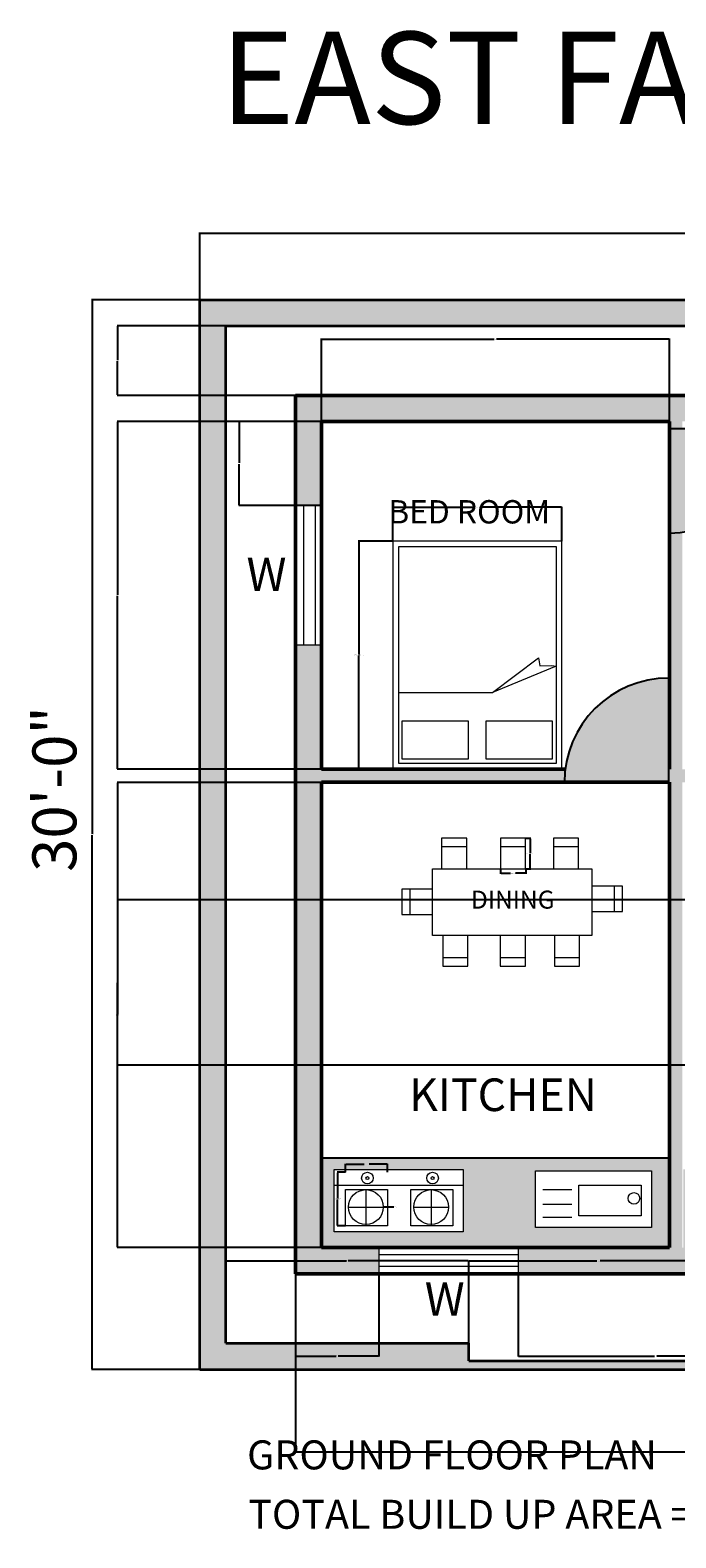
# Model space of a CAD drawing. Units: inches. Extents: x -48 to 546, y -53 to 467.
# Tile 1 of 3: x -48 to 174, y -53 to 467. Entities that reach past the tile are written whole.
import ezdxf

# ---------------------------------------------------------------- set-up
doc = ezdxf.new("R2010")
doc.units = ezdxf.units.IN
doc.header["$MEASUREMENT"] = 0
for name, color, linetype, lineweight in [('A-ANNO-DIMS', 2, 'Continuous', 18), ('A-ANNO-TEXT', 7, 'Continuous', 18), ('A-AREA-IDEN', 7, 'Continuous', 25), ('A-DOOR', 4, 'Continuous', 25), ('A-EQPM', 8, 'Continuous', 18), ('A-FLOR-CASE', 8, 'Continuous', 25), ('A-FLOR-FIXT', 9, 'Continuous', 18), ('A-FURN', 8, 'Continuous', 18), ('A-GLAZ', 4, 'Continuous', 18), ('A-WALL', 7, 'Continuous', 50), ('C-PROP', 7, 'Continuous', 35)]:
    doc.layers.add(name, color=color, linetype=linetype, lineweight=lineweight)
for name, color, linetype, lineweight, true_color in [('A-FLOR-PATT', 253, 'Continuous', 13, 0x9898cc), ('A-WALL-PATT', 251, 'Continuous', 13, 0x636466), ('C-PROP-PATT', 251, 'Continuous', 13, 0x636466)]:
    doc.layers.add(name, color=color, linetype=linetype, lineweight=lineweight, true_color=true_color)
doc.styles.get("Standard").update_dxf_attribs({"font": 'arial.ttf'})
doc.dimstyles.get("Standard").update_dxf_attribs({"dimtxt": 0.18, "dimasz": 0.18, "dimexe": 0.18, "dimexo": 0.0625, "dimgap": 0.09, "dimtad": 0, "dimtih": 1, "dimtoh": 1, "dimdec": 4, "dimzin": 0, "dimdsep": 46, "dimtxsty": 'Standard', "dimcen": 0.09, "dimadec": 0, "dimazin": 0, "dimtfac": 1, "dimtdec": 4, "dimtofl": 0, "dimtmove": 0, "dimatfit": 3, "dimfxl": 1, "dimtolj": 1, "dimtzin": 0, "dimarcsym": 0})

# ---------------------------------------------------------------- blocks, each defined once
blk = doc.blocks.new('*D3')
at = {"layer": 'A-ANNO-DIMS', "color": 0, "lineweight": -2, "transparency": 16777216}
for p, q in [((10.2, 374.58), (10.2, 397.68)), ((10.38, 397.5), (254.09, 397.5)), ((499.02, 397.5), (255.31, 397.5)), ((499.2, 374.58), (499.2, 397.68))]:
    blk.add_line(p, q, dxfattribs=at)
at = {"layer": 'A-ANNO-DIMS', "color": 0, "transparency": 16777216}
for points in [[(10.38, 397.53), (10.38, 397.47), (10.2, 397.5)], [(499.02, 397.53), (499.02, 397.47), (499.2, 397.5)]]:
    blk.add_solid(points, dxfattribs=at)
at = {"layer": 'Defpoints', "color": 0, "transparency": 16777216}
for p in [(499.2, 397.5), (10.2, 374.51), (499.2, 374.51)]:
    blk.add_point(p, dxfattribs=at)
at = {"layer": 'A-ANNO-DIMS', "color": 0, "transparency": 16777216, "insert": (254.7, 397.5), "char_height": 0.18, "width": 0.9058, "attachment_point": 5}
blk.add_mtext('\\A1;489.0000', dxfattribs=at)
blk = doc.blocks.new('*D4')
at = {"layer": 'A-ANNO-DIMS', "color": 0, "lineweight": -2, "transparency": 16777216}
for p, q in [((10.14, 374.51), (-27.18, 374.51)), ((-27, 374.33), (-27, 190.2)), ((-27, 5.69), (-27, 189.83)), ((10.14, 5.51), (-27.18, 5.51))]:
    blk.add_line(p, q, dxfattribs=at)
at = {"layer": 'A-ANNO-DIMS', "color": 0, "transparency": 16777216}
for points in [[(-27.03, 374.33), (-26.97, 374.33), (-27, 374.51)], [(-27.03, 5.69), (-26.97, 5.69), (-27, 5.51)]]:
    blk.add_solid(points, dxfattribs=at)
at = {"layer": 'Defpoints', "color": 0, "transparency": 16777216}
for p in [(10.2, 374.51), (-27, 5.51), (10.2, 5.51)]:
    blk.add_point(p, dxfattribs=at)
at = {"layer": 'A-ANNO-DIMS', "color": 0, "transparency": 16777216, "insert": (-27, 190.01), "char_height": 0.18, "attachment_point": 5}
blk.add_mtext('\\A1;369.0000', dxfattribs=at)
blk = doc.blocks.new('DOOR-SWING-36IN')
for p, q in [((0, 36), (0, 0)), ((0, 0), (36, 0))]:
    blk.add_line(p, q)
blk.add_arc((0, 0), 36, 0, 90)
blk = doc.blocks.new('CHAIR-DINING')
blk.add_line((0.01, 7.68), (8.69, 7.68))
blk.add_lwpolyline([(0, 0), (8.68, 0), (8.68, 10.53), (0, 10.53)], close=True)
blk = doc.blocks.new('BED-DOUBLE')
for p, q in [((34.35, 26.2), (50.2, 38.16)), ((50.2, 38.16), (50.65, 35.43)), ((56.35, 35.37), (34.37, 26.2)), ((50.65, 35.43), (54.7, 35.6)), ((1.91, 26.2), (34.35, 26.2))]:
    blk.add_line(p, q)
for points in [[(0, 0), (58.3, 0), (58.3, 78.39), (0, 78.39)], [(1.9, 1.9), (56.4, 1.9), (56.4, 76.49), (1.9, 76.49)], [(3.12, 3.4), (26.1, 3.4), (26.1, 16.4), (3.12, 16.4)], [(32.03, 3.4), (55.02, 3.4), (55.02, 16.4), (32.03, 16.4)]]:
    blk.add_lwpolyline(points, close=True)
blk = doc.blocks.new('WIN-48IN-FRONT')
for p, q in [((0, 9), (0, 0)), ((48, 6.49), (0, 6.49)), ((48, 9), (48, 0)), ((48, 2.49), (0, 2.49)), ((48, 2.49), (0, 2.49)), ((48, 2.49), (0, 2.49))]:
    blk.add_line(p, q)
blk = doc.blocks.new('WIN-48IN-BEDROOM')
for p, q in [((0, 48), (9, 48)), ((2.8, 48), (2.8, 0)), ((6.8, 48), (6.8, 0)), ((6.8, 48), (6.8, 0)), ((6.8, 48), (6.8, 0)), ((0, 0), (9, 0))]:
    blk.add_line(p, q)
blk = doc.blocks.new('COOKTOP-BURNER')
for p, q in [((7, 12.5), (7, 0)), ((1, 6.5), (13, 6.5))]:
    blk.add_line(p, q)
blk.add_lwpolyline([(0, 12.5), (14.5, 12.5), (14.5, 0), (0, 0)], close=True)
for centre, radius in [((7.5, 16.5), 2), ((7.5, 16.5), 0.5), ((7, 6.5), 6)]:
    blk.add_circle(centre, radius)
blk = doc.blocks.new('*D12')
at = {"layer": 'A-ANNO-DIMS', "color": 0, "lineweight": -2, "transparency": 16777216}
for p, q in [((76.76, 291.15), (64.88, 291.15)), ((65.06, 290.97), (65.06, 252.14)), ((65.06, 212.94), (65.06, 251.77)), ((76.76, 212.76), (64.88, 212.76))]:
    blk.add_line(p, q, dxfattribs=at)
at = {"layer": 'A-ANNO-DIMS', "color": 0, "transparency": 16777216}
for points in [[(65.03, 290.97), (65.09, 290.97), (65.06, 291.15)], [(65.03, 212.94), (65.09, 212.94), (65.06, 212.76)]]:
    blk.add_solid(points, dxfattribs=at)
at = {"layer": 'Defpoints', "color": 0, "transparency": 16777216}
for p in [(65.06, 291.15), (76.82, 291.15), (76.82, 212.76)]:
    blk.add_point(p, dxfattribs=at)
at = {"layer": 'A-ANNO-DIMS', "color": 0, "transparency": 16777216, "insert": (65.06, 251.95), "char_height": 0.18, "attachment_point": 5}
blk.add_mtext('\\A1;DOUBLE BED 6\'-6 1/2" TYP.', dxfattribs=at)
blk = doc.blocks.new('*D13')
at = {"layer": 'A-ANNO-DIMS', "color": 0, "lineweight": -2, "transparency": 16777216}
for p, q in [((76.82, 291.21), (76.82, 303.09)), ((77, 302.91), (105.05, 302.91)), ((134.94, 302.91), (106.89, 302.91)), ((135.12, 291.21), (135.12, 303.09))]:
    blk.add_line(p, q, dxfattribs=at)
at = {"layer": 'A-ANNO-DIMS', "color": 0, "transparency": 16777216}
for points in [[(77, 302.94), (77, 302.88), (76.82, 302.91)], [(134.94, 302.94), (134.94, 302.88), (135.12, 302.91)]]:
    blk.add_solid(points, dxfattribs=at)
at = {"layer": 'Defpoints', "color": 0, "transparency": 16777216}
for p in [(135.12, 302.91), (76.82, 291.15), (135.12, 291.15)]:
    blk.add_point(p, dxfattribs=at)
at = {"layer": 'A-ANNO-DIMS', "color": 0, "transparency": 16777216, "insert": (105.97, 302.91), "char_height": 0.18, "attachment_point": 5}
blk.add_mtext('\\A1;4\'-10 1/2" TYP.', dxfattribs=at)
blk = doc.blocks.new('*D22')
at = {"layer": 'A-ANNO-DIMS', "color": 0, "lineweight": -2, "transparency": 16777216}
for p, q in [((122.69, 188.75), (124.38, 188.75)), ((124.2, 188.57), (124.2, 183.67)), ((124.2, 178.4), (124.2, 183.3)), ((122.69, 178.22), (124.38, 178.22))]:
    blk.add_line(p, q, dxfattribs=at)
at = {"layer": 'A-ANNO-DIMS', "color": 0, "transparency": 16777216}
for points in [[(124.17, 188.57), (124.23, 188.57), (124.2, 188.75)], [(124.17, 178.4), (124.23, 178.4), (124.2, 178.22)]]:
    blk.add_solid(points, dxfattribs=at)
at = {"layer": 'Defpoints', "color": 0, "transparency": 16777216}
for p in [(122.63, 188.75), (124.2, 188.75), (122.63, 178.22)]:
    blk.add_point(p, dxfattribs=at)
at = {"layer": 'A-ANNO-DIMS', "color": 0, "transparency": 16777216, "insert": (124.2, 183.48), "char_height": 0.18, "attachment_point": 5}
blk.add_mtext('\\A1;CHAIR 0\'-10 1/2" TYP.', dxfattribs=at)
blk = doc.blocks.new('*D23')
at = {"layer": 'A-ANNO-DIMS', "color": 0, "lineweight": -2, "transparency": 16777216}
for p, q in [((113.94, 178.16), (113.94, 176.46)), ((122.63, 178.16), (122.63, 176.46)), ((114.12, 176.64), (117.43, 176.64)), ((122.45, 176.64), (119.13, 176.64))]:
    blk.add_line(p, q, dxfattribs=at)
at = {"layer": 'A-ANNO-DIMS', "color": 0, "transparency": 16777216}
for points in [[(114.12, 176.67), (114.12, 176.61), (113.94, 176.64)], [(122.45, 176.67), (122.45, 176.61), (122.63, 176.64)]]:
    blk.add_solid(points, dxfattribs=at)
at = {"layer": 'Defpoints', "color": 0, "transparency": 16777216}
for p in [(113.94, 178.22), (122.63, 178.22), (122.63, 176.64)]:
    blk.add_point(p, dxfattribs=at)
at = {"layer": 'A-ANNO-DIMS', "color": 0, "transparency": 16777216, "insert": (118.28, 176.64), "char_height": 0.18, "attachment_point": 5}
blk.add_mtext('\\A1;0\'-8 1/2" TYP.', dxfattribs=at)
blk = doc.blocks.new('*D24')
at = {"layer": 'A-ANNO-DIMS', "color": 0, "lineweight": -2, "transparency": 16777216}
for p, q in [((60.44, 73.5), (57.55, 73.5)), ((57.73, 73.32), (57.73, 64.43)), ((57.73, 55.18), (57.73, 64.07)), ((60.44, 55), (57.55, 55))]:
    blk.add_line(p, q, dxfattribs=at)
at = {"layer": 'A-ANNO-DIMS', "color": 0, "transparency": 16777216}
for points in [[(57.7, 73.32), (57.76, 73.32), (57.73, 73.5)], [(57.7, 55.18), (57.76, 55.18), (57.73, 55)]]:
    blk.add_solid(points, dxfattribs=at)
at = {"layer": 'Defpoints', "color": 0, "transparency": 16777216}
for p in [(57.73, 73.5), (60.5, 73.5), (60.5, 55)]:
    blk.add_point(p, dxfattribs=at)
at = {"layer": 'A-ANNO-DIMS', "color": 0, "transparency": 16777216, "insert": (57.73, 64.25), "char_height": 0.18, "attachment_point": 5}
blk.add_mtext('\\A1;BURNER 1\'-6 1/2" TYP.', dxfattribs=at)
blk = doc.blocks.new('*D25')
at = {"layer": 'A-ANNO-DIMS', "color": 0, "lineweight": -2, "transparency": 16777216}
for p, q in [((60.5, 73.56), (60.5, 76.46)), ((60.68, 76.28), (66.91, 76.28)), ((74.82, 76.28), (68.59, 76.28)), ((75, 73.56), (75, 76.46))]:
    blk.add_line(p, q, dxfattribs=at)
at = {"layer": 'A-ANNO-DIMS', "color": 0, "transparency": 16777216}
for points in [[(60.68, 76.31), (60.68, 76.25), (60.5, 76.28)], [(74.82, 76.31), (74.82, 76.25), (75, 76.28)]]:
    blk.add_solid(points, dxfattribs=at)
at = {"layer": 'Defpoints', "color": 0, "transparency": 16777216}
for p in [(60.5, 73.5), (75, 76.28), (75, 73.5)]:
    blk.add_point(p, dxfattribs=at)
at = {"layer": 'A-ANNO-DIMS', "color": 0, "transparency": 16777216, "insert": (67.75, 76.28), "char_height": 0.18, "attachment_point": 5}
blk.add_mtext('\\A1;1\'-2 1/2" TYP.', dxfattribs=at)
blk = doc.blocks.new('*D26')
at = {"layer": 'A-ANNO-DIMS', "color": 0, "lineweight": -2, "transparency": 16777216}
for p, q in [((43.2, 38.45), (43.2, -23.08)), ((466.2, 38.45), (466.2, -23.08)), ((43.38, -22.9), (254.3, -22.9)), ((466.02, -22.9), (255.1, -22.9))]:
    blk.add_line(p, q, dxfattribs=at)
at = {"layer": 'A-ANNO-DIMS', "color": 0, "transparency": 16777216}
for points in [[(43.38, -22.87), (43.38, -22.93), (43.2, -22.9)], [(466.02, -22.87), (466.02, -22.93), (466.2, -22.9)]]:
    blk.add_solid(points, dxfattribs=at)
at = {"layer": 'Defpoints', "color": 0, "transparency": 16777216}
for p in [(43.2, 38.51), (466.2, 38.51), (466.2, -22.9)]:
    blk.add_point(p, dxfattribs=at)
at = {"layer": 'A-ANNO-DIMS', "color": 0, "transparency": 16777216, "insert": (254.7, -22.9), "char_height": 0.18, "attachment_point": 5}
blk.add_mtext('\\A1;35\'-3"', dxfattribs=at)
blk = doc.blocks.new('*D29')
at = {"layer": 'A-ANNO-DIMS', "color": 0, "lineweight": -2, "transparency": 16777216}
for p, q in [((19.14, 365.51), (-18.38, 365.51)), ((-18.2, 365.33), (-18.2, 353.7)), ((-18.2, 341.69), (-18.2, 353.33)), ((43.14, 341.51), (-18.38, 341.51))]:
    blk.add_line(p, q, dxfattribs=at)
at = {"layer": 'A-ANNO-DIMS', "color": 0, "transparency": 16777216}
for points in [[(-18.23, 365.33), (-18.17, 365.33), (-18.2, 365.51)], [(-18.23, 341.69), (-18.17, 341.69), (-18.2, 341.51)]]:
    blk.add_solid(points, dxfattribs=at)
at = {"layer": 'Defpoints', "color": 0, "transparency": 16777216}
for p in [(19.2, 365.51), (-18.2, 341.51), (43.2, 341.51)]:
    blk.add_point(p, dxfattribs=at)
at = {"layer": 'A-ANNO-DIMS', "color": 0, "transparency": 16777216, "insert": (-18.2, 353.51), "char_height": 0.18, "attachment_point": 5}
blk.add_mtext('\\A1;2\'-0"', dxfattribs=at)
blk = doc.blocks.new('*D30')
at = {"layer": 'A-ANNO-DIMS', "color": 0, "lineweight": -2, "transparency": 16777216}
for p, q in [((52.2, 332.58), (52.2, 361.09)), ((52.38, 360.91), (111.81, 360.91)), ((172.02, 360.91), (112.59, 360.91)), ((172.2, 332.58), (172.2, 361.09))]:
    blk.add_line(p, q, dxfattribs=at)
at = {"layer": 'A-ANNO-DIMS', "color": 0, "transparency": 16777216}
for points in [[(52.38, 360.94), (52.38, 360.88), (52.2, 360.91)], [(172.02, 360.94), (172.02, 360.88), (172.2, 360.91)]]:
    blk.add_solid(points, dxfattribs=at)
at = {"layer": 'Defpoints', "color": 0, "transparency": 16777216}
for p in [(172.2, 360.91), (52.2, 332.51), (172.2, 332.51)]:
    blk.add_point(p, dxfattribs=at)
at = {"layer": 'A-ANNO-DIMS', "color": 0, "transparency": 16777216, "insert": (112.2, 360.91), "char_height": 0.18, "attachment_point": 5}
blk.add_mtext('\\A1;10\'-0"', dxfattribs=at)
blk = doc.blocks.new('*D34')
at = {"layer": 'A-ANNO-DIMS', "color": 0, "lineweight": -2, "transparency": 16777216}
for p, q in [((52.14, 332.51), (-18.38, 332.51)), ((-18.2, 332.33), (-18.2, 272.7)), ((-18.2, 212.69), (-18.2, 272.33)), ((52.14, 212.51), (-18.38, 212.51))]:
    blk.add_line(p, q, dxfattribs=at)
at = {"layer": 'A-ANNO-DIMS', "color": 0, "transparency": 16777216}
for points in [[(-18.23, 332.33), (-18.17, 332.33), (-18.2, 332.51)], [(-18.23, 212.69), (-18.17, 212.69), (-18.2, 212.51)]]:
    blk.add_solid(points, dxfattribs=at)
at = {"layer": 'Defpoints', "color": 0, "transparency": 16777216}
for p in [(-18.2, 332.51), (52.2, 332.51), (52.2, 212.51)]:
    blk.add_point(p, dxfattribs=at)
at = {"layer": 'A-ANNO-DIMS', "color": 0, "transparency": 16777216, "insert": (-18.2, 272.51), "char_height": 0.18, "attachment_point": 5}
blk.add_mtext('\\A1;10\'-0"', dxfattribs=at)
blk = doc.blocks.new('*D35')
at = {"layer": 'A-ANNO-DIMS', "color": 0, "lineweight": -2, "transparency": 16777216}
for p, q in [((52.14, 208.01), (-18.38, 208.01)), ((-18.2, 207.83), (-18.2, 127.95)), ((-18.2, 47.69), (-18.2, 127.58)), ((52.14, 47.51), (-18.38, 47.51))]:
    blk.add_line(p, q, dxfattribs=at)
at = {"layer": 'A-ANNO-DIMS', "color": 0, "transparency": 16777216}
for points in [[(-18.23, 207.83), (-18.17, 207.83), (-18.2, 208.01)], [(-18.23, 47.69), (-18.17, 47.69), (-18.2, 47.51)]]:
    blk.add_solid(points, dxfattribs=at)
at = {"layer": 'Defpoints', "color": 0, "transparency": 16777216}
for p in [(-18.2, 208.01), (52.2, 208.01), (52.2, 47.51)]:
    blk.add_point(p, dxfattribs=at)
at = {"layer": 'A-ANNO-DIMS', "color": 0, "transparency": 16777216, "insert": (-18.2, 127.76), "char_height": 0.18, "attachment_point": 5}
blk.add_mtext('\\A1;13\'-4 1/2"', dxfattribs=at)
blk = doc.blocks.new('*D40')
at = {"layer": 'A-ANNO-DIMS', "color": 0, "lineweight": -2, "transparency": 16777216}
for p, q in [((43.2, 38.45), (43.2, 9.93)), ((72, 38.45), (72, 9.93)), ((43.38, 10.11), (57.27, 10.11)), ((71.82, 10.11), (57.93, 10.11))]:
    blk.add_line(p, q, dxfattribs=at)
at = {"layer": 'A-ANNO-DIMS', "color": 0, "transparency": 16777216}
for points in [[(43.38, 10.14), (43.38, 10.08), (43.2, 10.11)], [(71.82, 10.14), (71.82, 10.08), (72, 10.11)]]:
    blk.add_solid(points, dxfattribs=at)
at = {"layer": 'Defpoints', "color": 0, "transparency": 16777216}
for p in [(43.2, 38.51), (72, 38.51), (43.2, 10.11)]:
    blk.add_point(p, dxfattribs=at)
at = {"layer": 'A-ANNO-DIMS', "color": 0, "transparency": 16777216, "insert": (57.6, 10.11), "char_height": 0.18, "attachment_point": 5}
blk.add_mtext('\\A1;2\'-5"', dxfattribs=at)
blk = doc.blocks.new('*D41')
at = {"layer": 'A-ANNO-DIMS', "color": 0, "lineweight": -2, "transparency": 16777216}
for p, q in [((120, 38.45), (120, 9.93)), ((215, 38.45), (215, 9.93)), ((120.18, 10.11), (167.1, 10.11)), ((214.82, 10.11), (167.9, 10.11))]:
    blk.add_line(p, q, dxfattribs=at)
at = {"layer": 'A-ANNO-DIMS', "color": 0, "transparency": 16777216}
for points in [[(120.18, 10.14), (120.18, 10.08), (120, 10.11)], [(214.82, 10.14), (214.82, 10.08), (215, 10.11)]]:
    blk.add_solid(points, dxfattribs=at)
at = {"layer": 'Defpoints', "color": 0, "transparency": 16777216}
for p in [(120, 38.51), (215, 38.51), (120, 10.11)]:
    blk.add_point(p, dxfattribs=at)
at = {"layer": 'A-ANNO-DIMS', "color": 0, "transparency": 16777216, "insert": (167.5, 10.11), "char_height": 0.18, "attachment_point": 5}
blk.add_mtext('\\A1;7\'-11"', dxfattribs=at)
blk = doc.blocks.new('*D42')
at = {"layer": 'A-ANNO-DIMS', "color": 0, "lineweight": -2, "transparency": 16777216}
for p, q in [((52.14, 332.51), (23.62, 332.51)), ((23.8, 332.33), (23.8, 318.19)), ((23.8, 303.68), (23.8, 317.82)), ((52.14, 303.5), (23.62, 303.5))]:
    blk.add_line(p, q, dxfattribs=at)
at = {"layer": 'A-ANNO-DIMS', "color": 0, "transparency": 16777216}
for points in [[(23.77, 332.33), (23.83, 332.33), (23.8, 332.51)], [(23.77, 303.68), (23.83, 303.68), (23.8, 303.5)]]:
    blk.add_solid(points, dxfattribs=at)
at = {"layer": 'Defpoints', "color": 0, "transparency": 16777216}
for p in [(23.8, 332.51), (52.2, 332.51), (52.2, 303.5)]:
    blk.add_point(p, dxfattribs=at)
at = {"layer": 'A-ANNO-DIMS', "color": 0, "transparency": 16777216, "insert": (23.8, 318.01), "char_height": 0.18, "attachment_point": 5}
blk.add_mtext('\\A1;2\'-5"', dxfattribs=at)
blk = doc.blocks.new('*D45')
at = {"layer": 'A-ANNO-DIMS', "color": 0, "lineweight": -2, "transparency": 16777216}
for p, q in [((456.95, 167.5), (-18.38, 167.5)), ((-18.2, 167.32), (-18.2, 139.18)), ((-18.2, 110.68), (-18.2, 138.82)), ((457.14, 110.5), (-18.38, 110.5))]:
    blk.add_line(p, q, dxfattribs=at)
at = {"layer": 'A-ANNO-DIMS', "color": 0, "transparency": 16777216}
for points in [[(-18.23, 167.32), (-18.17, 167.32), (-18.2, 167.5)], [(-18.23, 110.68), (-18.17, 110.68), (-18.2, 110.5)]]:
    blk.add_solid(points, dxfattribs=at)
at = {"layer": 'Defpoints', "color": 0, "transparency": 16777216}
for p in [(457.01, 167.5), (-18.2, 110.5), (457.2, 110.5)]:
    blk.add_point(p, dxfattribs=at)
at = {"layer": 'A-ANNO-DIMS', "color": 0, "transparency": 16777216, "insert": (-18.2, 139), "char_height": 0.18, "attachment_point": 5}
blk.add_mtext('\\A1;4\'-9"', dxfattribs=at)
blk = doc.blocks.new('*D49')
at = {"layer": 'A-ANNO-DIMS', "color": 0, "lineweight": -2, "transparency": 16777216}
for p, q in [((103, 14.58), (103, 43.09)), ((103.18, 42.91), (147.21, 42.91)), ((192.32, 42.91), (148.29, 42.91)), ((192.5, 14.58), (192.5, 43.09))]:
    blk.add_line(p, q, dxfattribs=at)
at = {"layer": 'A-ANNO-DIMS', "color": 0, "transparency": 16777216}
for points in [[(103.18, 42.94), (103.18, 42.88), (103, 42.91)], [(192.32, 42.94), (192.32, 42.88), (192.5, 42.91)]]:
    blk.add_solid(points, dxfattribs=at)
at = {"layer": 'Defpoints', "color": 0, "transparency": 16777216}
for p in [(192.5, 42.91), (103, 14.51), (192.5, 14.51)]:
    blk.add_point(p, dxfattribs=at)
at = {"layer": 'A-ANNO-DIMS', "color": 0, "transparency": 16777216, "insert": (147.75, 42.91), "char_height": 0.18, "attachment_point": 5}
blk.add_mtext('\\A1;7\'-5 1/2"', dxfattribs=at)
blk = doc.blocks.new('*D50')
at = {"layer": 'A-ANNO-DIMS', "color": 0, "lineweight": -2, "transparency": 16777216}
for p, q in [((19.2, 14.58), (19.2, 43.09)), ((19.38, 42.91), (60.77, 42.91)), ((102.82, 42.91), (61.43, 42.91)), ((103, 14.58), (103, 43.09))]:
    blk.add_line(p, q, dxfattribs=at)
at = {"layer": 'A-ANNO-DIMS', "color": 0, "transparency": 16777216}
for points in [[(19.38, 42.94), (19.38, 42.88), (19.2, 42.91)], [(102.82, 42.94), (102.82, 42.88), (103, 42.91)]]:
    blk.add_solid(points, dxfattribs=at)
at = {"layer": 'Defpoints', "color": 0, "transparency": 16777216}
for p in [(103, 42.91), (19.2, 14.51), (103, 14.51)]:
    blk.add_point(p, dxfattribs=at)
at = {"layer": 'A-ANNO-DIMS', "color": 0, "transparency": 16777216, "insert": (61.1, 42.91), "char_height": 0.18, "attachment_point": 5}
blk.add_mtext('\\A1;7\'-0"', dxfattribs=at)
blk = doc.blocks.new('*D52')
at = {"layer": 'A-ANNO-DIMS', "color": 0, "lineweight": -2, "transparency": 16777216}
for p, q in [((67.41, 61.5), (67.59, 61.5)), ((67.5, 61.41), (67.5, 61.59)), ((77.1, 61.5), (73.68, 61.5))]:
    blk.add_line(p, q, dxfattribs=at)
at = {"layer": 'A-ANNO-DIMS', "color": 0, "transparency": 16777216}
blk.add_solid([(73.68, 61.53), (73.68, 61.47), (73.5, 61.5)], dxfattribs=at)
at = {"layer": 'Defpoints', "color": 0, "transparency": 16777216}
for p in [(61.5, 61.5), (73.5, 61.5)]:
    blk.add_point(p, dxfattribs=at)
at = {"layer": 'A-ANNO-DIMS', "color": 0, "transparency": 16777216, "insert": (77.72, 61.5), "char_height": 0.18, "attachment_point": 5}
blk.add_mtext('\\A1;2X ∅1\'-0"', dxfattribs=at)

msp = doc.modelspace()

# ---------------------------------------------------------------- hatches: boundary and pattern name
at = {"layer": 'A-FLOR-PATT'}
h = msp.add_hatch(color=256, dxfattribs=at)
h.dxf.hatch_style = 1
h.paths.add_polyline_path([(208.19994, 330.01344), (172.19994, 330.01344), (172.19994, 294.01344, 0.414213549)])
h.paths.add_polyline_path([(320.5, 332.5), (284.5, 332.5, 0.414213562), (320.5, 296.5)])
h.paths.add_polyline_path([(417, 204.5), (381, 204.5), (381, 168.5, 0.414213562)])
h.paths.add_polyline_path([(177, 74.5), (177, 38.51344), (213, 38.51344, 0.414104244)])
h.paths.add_polyline_path([(172, 244, 0.414104258), (136, 208.01344), (172, 208.01344)])
h.paths.add_polyline_path([(320.69994, 244.01344), (320.69994, 212.51344), (320.69994, 208.01344), (356.69994, 208.01344, 0.414213532)])
h.paths.add_polyline_path([(172.19994, 78.5), (52.19994, 78.5), (52.19994, 47.51344), (172.19994, 47.51344)])
h.paths.add_polyline_path([(126, 74), (166, 74), (166, 54.5), (126, 54.5)], flags=16)
h.paths.add_polyline_path([(101, 53), (56.5, 53), (56.5, 74.5), (101, 74.5)], flags=16)
h.paths.add_polyline_path([(141, 69), (162.5, 69), (162.5, 58.5), (141, 58.5)], flags=0)
h.paths.add_polyline_path([(97.5, 55), (83, 55), (83, 67.5), (97.5, 67.5)], flags=0)
h.paths.add_polyline_path([(84, 61.5, -1), (96, 61.5, -1)], flags=0)
h.paths.add_polyline_path([(88.5, 71.5, -1), (92.5, 71.5, -1)], flags=0)
h.paths.add_polyline_path([(90, 71.5, -1), (91, 71.5, -1)], flags=0)
h.paths.add_polyline_path([(162, 64.5, -1), (158, 64.5, -1)], flags=0)
h.paths.add_polyline_path([(75, 55), (60.5, 55), (60.5, 67.5), (75, 67.5)], flags=0)
h.paths.add_polyline_path([(61.5, 61.5, -1), (73.5, 61.5, -1)], flags=0)
h.paths.add_polyline_path([(66, 71.5, -1), (70, 71.5, -1)], flags=0)
h.paths.add_polyline_path([(67.5, 71.5, -1), (68.5, 71.5, -1)], flags=0)
h.paths.add_polyline_path([(176.42827, 40.63764), (207.16292, 40.63764), (207.16292, 57.88764), (176.42827, 57.88764)], flags=9)
at = {"layer": 'A-WALL-PATT'}
h = msp.add_hatch(color=256, dxfattribs=at)
h.dxf.hatch_style = 1
h.paths.add_polyline_path([(282.44994, 341.51344), (234.44994, 341.51344), (234.44994, 332.51344), (244.19994, 332.51344), (244.19994, 212.51344), (176.69994, 212.51344), (176.69994, 294.29579, -0.031342215), (172.19994, 294.01344), (172.19994, 212.51344), (172.00059, 208.01344), (172.19994, 208.01344), (172.19994, 47.51344), (120, 47.51344), (120, 38.51344), (177, 38.51344), (177, 47.51344), (176.69994, 47.51344), (176.69994, 208.01344), (320.69994, 208.01344), (320.69994, 244.01344), (320.69994, 296.50056, -0.031331714), (316.19994, 296.75774), (316.19994, 212.51344), (248.69994, 212.51344), (248.69994, 332.51344), (282.44994, 332.51344)])
h.paths.add_polyline_path([(466.19994, 341.51344), (306.44994, 341.51344), (306.44994, 332.51344), (316.19994, 332.51344), (457.19994, 332.51344), (457.19994, 304.5), (466.19994, 304.5)])
h.paths.add_polyline_path([(466.19994, 256.5), (457.19994, 256.5), (457.19994, 212.51344), (423.64319, 212.51344), (423.64319, 212.34928), (365.34701, 212.34928), (356.41758, 212.51344, -0.031342215), (356.69994, 208.01344), (380.69994, 208.01344), (380.69994, 204.5), (385.19994, 204.5), (385.19994, 208.01344), (457.19994, 208.01344), (457.19994, 191.5), (466.19994, 191.5)])
h.paths.add_polyline_path([(210.44994, 341.51344), (43.19994, 341.51344), (43.19994, 303.5), (52.19994, 303.5), (52.19994, 332.51344), (172.19994, 332.51344), (172.19994, 330.01344), (176.69994, 330.01344), (176.69994, 332.51344), (210.44994, 332.51344)])
h.paths.add_polyline_path([(52.19994, 208.01344), (136, 208.01344, -0.031342955), (136.28405, 212.51344), (52.19994, 212.51344), (52.19994, 255.5), (43.19994, 255.5), (43.19994, 38.51344), (72, 38.51344), (72, 47.51344), (52.19994, 47.51344)])
h.paths.add_polyline_path([(466.19994, 62.5), (457.19994, 62.5), (457.19994, 47.51344), (380.69994, 47.51344), (263, 47.51344), (263, 38.51344), (466.19994, 38.51344)])
h.paths.add_polyline_path([(215, 47.51344), (211.85338, 47.51344, -0.063257301), (213, 38.51344), (215, 38.51344)])
h.paths.add_polyline_path([(466.19994, 167.5), (457.19994, 167.5), (457.19994, 136.01344), (385.19994, 136.01344), (385.19994, 168.74583, -0.031326837), (380.69994, 168.50125), (380.69994, 131.51344), (457.19994, 131.51344), (457.19994, 110.5), (466.19994, 110.5)])
h = msp.add_hatch(color=256, dxfattribs=at)
h.dxf.hatch_style = 1
h.paths.add_polyline_path([(210.44994, 341.51344), (43.19994, 341.51344), (43.19994, 303.5), (52.19994, 303.5), (52.19994, 332.51344), (172.19994, 332.51344), (172.19994, 330.01344), (176.69994, 330.01344), (176.69994, 332.51344), (210.44994, 332.51344)])
h.paths.add_polyline_path([(466.19994, 341.51344), (306.44994, 341.51344), (306.44994, 332.51344), (316.19994, 332.51344), (457.19994, 332.51344), (457.19994, 304.5), (466.19994, 304.5)])
h.paths.add_polyline_path([(282.44994, 341.51344), (234.44994, 341.51344), (234.44994, 332.51344), (244.19994, 332.51344), (244.19994, 212.51344), (176.69994, 212.51344), (176.69994, 294.29579, -0.031342215), (172.19994, 294.01344), (172.19994, 212.51344), (172.00059, 208.01344), (172.19994, 208.01344), (172.19994, 47.51344), (120, 47.51344), (120, 38.51344), (177, 38.51344), (177, 47.51344), (176.69994, 47.51344), (176.69994, 208.01344), (320.69994, 208.01344), (320.69994, 244.01344), (320.69994, 296.50056, -0.031331714), (316.19994, 296.75774), (316.19994, 212.51344), (248.69994, 212.51344), (248.69994, 332.51344), (282.44994, 332.51344)])
h.paths.add_polyline_path([(52.19994, 255.5), (43.19994, 255.5), (43.19994, 38.51344), (72, 38.51344), (72, 47.51344), (52.19994, 47.51344), (52.19994, 208.01344), (136, 208.01344, -0.031342955), (136.28405, 212.51344), (52.19994, 212.51344)])
h.paths.add_polyline_path([(466.19994, 256.5), (457.19994, 256.5), (457.19994, 212.51344), (423.64319, 212.51344), (423.64319, 212.34928), (365.34701, 212.34928), (356.41758, 212.51344, -0.031342215), (356.69994, 208.01344), (380.69994, 208.01344), (380.69994, 204.5), (385.19994, 204.5), (385.19994, 208.01344), (457.19994, 208.01344), (457.19994, 191.5), (466.19994, 191.5)])
h.paths.add_polyline_path([(466.19994, 167.5), (457.19994, 167.5), (457.19994, 136.01344), (385.19994, 136.01344), (385.19994, 168.74583, -0.031326837), (380.69994, 168.50125), (380.69994, 131.51344), (457.19994, 131.51344), (457.19994, 110.5), (466.19994, 110.5)])
h.paths.add_polyline_path([(466.19994, 62.5), (457.19994, 62.5), (457.19994, 47.51344), (380.69994, 47.51344), (263, 47.51344), (263, 38.51344), (466.19994, 38.51344)])
h.paths.add_polyline_path([(215, 47.51344), (211.85338, 47.51344, -0.063257301), (213, 38.51344), (215, 38.51344)])
at = {"layer": 'C-PROP-PATT'}
h = msp.add_hatch(color=256, dxfattribs=at)
h.dxf.hatch_style = 1
h.paths.add_polyline_path([(499.19994, 374.51344), (10.19994, 374.51344), (10.19994, 5.51344), (103, 5.51344), (103, 14.51344), (19.19994, 14.51344), (19.19994, 365.51344), (490.19994, 365.51344), (490.19994, 14.51344), (192.5, 14.51344), (192.5, 5.51344), (499.19994, 5.51344)])
h = msp.add_hatch(color=256, dxfattribs=at)
h.dxf.hatch_style = 1
h.paths.add_polyline_path([(192.5, 8.5), (103, 8.5), (103, 5.5), (192.5, 5.5)])

# ---------------------------------------------------------------- linework, layer by layer
at = {"layer": 'A-EQPM'}
msp.add_line((56.5, 69), (101, 69), dxfattribs=at)
msp.add_lwpolyline([(56.5, 74.5), (101, 74.5), (101, 53), (56.5, 53)], close=True, dxfattribs=at)
at = {"layer": 'A-FLOR-CASE'}
msp.add_line((52, 78.5), (172, 78.5), dxfattribs=at)
at = {"layer": 'A-FLOR-FIXT'}
for p, q in [((128.5, 67.5), (138.5, 67.5)), ((128.5, 62.5), (138.5, 62.5)), ((128.5, 58), (138.5, 58))]:
    msp.add_line(p, q, dxfattribs=at)
for points in [[(126, 74), (166, 74), (166, 54.5), (126, 54.5)], [(141, 69), (162.5, 69), (162.5, 58.5), (141, 58.5)]]:
    msp.add_lwpolyline(points, close=True, dxfattribs=at)
msp.add_circle((160, 64.5), 2, dxfattribs=at)
at = {"layer": 'A-FURN'}
msp.add_line((131.52139, 248.36108), (133.17459, 248.13326), dxfattribs=at)
msp.add_lwpolyline([(90.45471, 178.21012), (145.49796, 178.21012), (145.49796, 155.14263), (90.45471, 155.14263)], close=True, dxfattribs=at)
at = {"layer": 'A-WALL'}
for p, q in [((43.19994, 38.51344), (43.19994, 341.51344)), ((43.19994, 341.51344), (466.19994, 341.51344)), ((52.19994, 332.51344), (172.19994, 332.51344)), ((52.19994, 212.51344), (52.19994, 332.51344)), ((172.19994, 212.51344), (172.19994, 332.51344)), ((52.19994, 212.51344), (136.28405, 212.51344)), ((172, 212.51344), (172.19994, 212.51344)), ((52.19994, 47.51344), (52.19994, 208.01344)), ((52.19994, 208.01344), (172.19994, 208.01344)), ((172.19994, 47.51344), (172.19994, 208.01344)), ((52.19994, 47.51344), (172.19994, 47.51344)), ((43.19994, 38.51344), (466.19994, 38.51344))]:
    msp.add_line(p, q, dxfattribs=at)
at = {"layer": 'C-PROP'}
for p, q in [((10.19994, 5.51344), (10.19994, 374.51344)), ((10.19994, 374.51344), (499.19994, 374.51344)), ((19.19994, 365.51344), (490.19994, 365.51344)), ((19.19994, 14.51344), (19.19994, 365.51344)), ((19.19994, 14.51344), (103, 14.51344)), ((10.19994, 5.51344), (103, 5.51344)), ((103, 8.5), (192.5, 8.5)), ((103, 5.5), (192.5, 5.5))]:
    msp.add_line(p, q, dxfattribs=at)
for points in [[(103, 8.5), (103, 14.51344)], [(103, 5.5), (103, 5.51344)]]:
    msp.add_lwpolyline(points, dxfattribs=at)

# ---------------------------------------------------------------- block references
at = {"layer": 'A-DOOR'}
for p, rotation in [((172.19951, 330.01338), 270.0000000000002), ((172.00043, 208.00006), 89.99999999999994)]:
    msp.add_blockref('DOOR-SWING-36IN', p, dxfattribs=dict(at, rotation=rotation))
at = {"layer": 'A-EQPM'}
for p in [(60.5, 55), (83, 55)]:
    msp.add_blockref('COOKTOP-BURNER', p, dxfattribs=at)
at = {"layer": 'A-FURN'}
for name, p in [('BED-DOUBLE', (76.82, 212.761)), ('CHAIR-DINING', (93.634, 178.218)), ('CHAIR-DINING', (113.93878, 178.218)), ('CHAIR-DINING', (132.21308, 178.218))]:
    msp.add_blockref(name, p, dxfattribs=at)
for p, rotation in [((145.45668, 172.14864), 270.0000000000003), ((90.45703, 162.46325), 90.0000000000003), ((102.71903, 155.14861), 180), ((122.52885, 155.14861), 180), ((141.25319, 155.14861), 180)]:
    msp.add_blockref('CHAIR-DINING', p, dxfattribs=dict(at, rotation=rotation))
at = {"layer": 'A-GLAZ'}
for name, p in [('WIN-48IN-BEDROOM', (43.2, 255.5)), ('WIN-48IN-FRONT', (72, 38.513))]:
    msp.add_blockref(name, p, dxfattribs=at)

# ---------------------------------------------------------------- texts
at = {"layer": 'A-ANNO-DIMS'}
msp.add_text('30\'-0"', height=15.166687, rotation=90, dxfattribs=at).set_placement((-32.41276, 177.11293))
at = {"layer": 'A-ANNO-TEXT'}
for s, height, p in [('EAST FACING HOUSE', 31.8325196, (17.25357, 435.09398)), ('W', 11.5, (26.30327, 274.01264)), ('W', 11.5, (87.80327, 24.01264)), ('GROUND FLOOR PLAN', 10, (26.5, -29)), ('TOTAL BUILD UP AREA = 1200sqft', 10, (26.91088, -49.49293))]:
    msp.add_text(s, height=height, dxfattribs=at).set_placement(p)
at = {"layer": 'A-AREA-IDEN'}
for s, height, p in [('BED ROOM', 8.042128, (75.22343, 297.31708)), ('DINING', 6.200411, (103.75463, 164.44636)), ('KITCHEN', 11.2677, (82.40665, 94.60168))]:
    msp.add_text(s, height=height, dxfattribs=at).set_placement(p)

# ---------------------------------------------------------------- dimensions: what is measured, and where the dimension line sits
at = {"layer": 'A-ANNO-DIMS'}
for base, p1, p2, override, picture, middle in [((499.19994, 397.5), (10.19994, 374.51344), (499.19994, 374.51344), {"dimclrd": 0, "dimclre": 0, "dimclrt": 0}, '*D3', (254.69994, 397.5)), ((172.19994, 360.91344), (52.19994, 332.51344), (172.19994, 332.51344), {"dimdec": 1, "dimlfac": 1, "dimrnd": 0, "dimzin": 1, "dimdsep": 46, "dimlunit": 4, "dimfrac": 2}, '*D30', (112.19994, 360.91344)), ((103, 42.91344), (19.19994, 14.51344), (103, 14.51344), {"dimdec": 1, "dimlfac": 1, "dimrnd": 0, "dimzin": 1, "dimdsep": 46, "dimlunit": 4, "dimfrac": 2}, '*D50', (61.09997, 42.91344)), ((192.5, 42.91344), (103, 14.51344), (192.5, 14.51344), {"dimdec": 1, "dimlfac": 1, "dimrnd": 0, "dimzin": 1, "dimdsep": 46, "dimlunit": 4, "dimfrac": 2}, '*D49', (147.75, 42.91344)), ((466.19994, -22.9), (43.19994, 38.51344), (466.19994, 38.51344), {"dimdec": 1, "dimlfac": 1, "dimrnd": 0, "dimzin": 1, "dimdsep": 46, "dimlunit": 4, "dimfrac": 2}, '*D26', (254.69994, -22.9))]:
    dim = msp.add_linear_dim(base=base, p1=p1, p2=p2, dimstyle='Standard', override=override, dxfattribs=at)
    dim.commit()
    dim.dimension.update_dxf_attribs({"geometry": picture, "text_midpoint": middle})
for base, p1, p2, angle, override, picture, middle in [((-27, 5.51344), (10.19994, 374.51344), (10.19994, 5.51344), 90, {"dimclrd": 0, "dimclre": 0, "dimclrt": 0}, '*D4', (-27, 190.01344)), ((-18.20006, 341.51344), (19.19994, 365.51344), (43.19994, 341.51344), 90, {"dimdec": 1, "dimlfac": 1, "dimrnd": 0, "dimzin": 1, "dimdsep": 46, "dimlunit": 4, "dimfrac": 2}, '*D29', (-18.20006, 353.51344)), ((-18.20006, 332.51344), (52.19994, 212.51344), (52.19994, 332.51344), 90, {"dimdec": 1, "dimlfac": 1, "dimrnd": 0, "dimzin": 1, "dimdsep": 46, "dimlunit": 4, "dimfrac": 2}, '*D34', (-18.20006, 272.51344)), ((23.79994, 332.51344), (52.19994, 303.5), (52.19994, 332.51344), 90, {"dimdec": 1, "dimlfac": 1, "dimrnd": 0, "dimzin": 1, "dimdsep": 46, "dimlunit": 4, "dimfrac": 2}, '*D42', (23.79994, 318.00672)), ((-18.20006, 208.01344), (52.19994, 47.51344), (52.19994, 208.01344), 90, {"dimdec": 1, "dimlfac": 1, "dimrnd": 0, "dimzin": 1, "dimdsep": 46, "dimlunit": 4, "dimfrac": 2}, '*D35', (-18.20006, 127.76344)), ((-18.20006, 110.5), (457.01404, 167.5), (457.19994, 110.5), 90, {"dimdec": 1, "dimlfac": 1, "dimrnd": 0, "dimzin": 1, "dimdsep": 46, "dimlunit": 4, "dimfrac": 2}, '*D45', (-18.20006, 139)), ((43.19994, 10.11344), (72, 38.51344), (43.19994, 38.51344), 180, {"dimdec": 1, "dimlfac": 1, "dimrnd": 0, "dimzin": 1, "dimdsep": 46, "dimlunit": 4, "dimfrac": 2}, '*D40', (57.59997, 10.11344)), ((120, 10.11344), (215, 38.51344), (120, 38.51344), 180, {"dimdec": 1, "dimlfac": 1, "dimrnd": 0, "dimzin": 1, "dimdsep": 46, "dimlunit": 4, "dimfrac": 2}, '*D41', (167.5, 10.11344))]:
    dim = msp.add_linear_dim(base=base, p1=p1, p2=p2, angle=angle, dimstyle='Standard', override=override, dxfattribs=at)
    dim.commit()
    dim.dimension.update_dxf_attribs({"geometry": picture, "text_midpoint": middle})
for base, p1, p2, picture, middle in [((135.11617, 302.9062), (76.81999, 291.14809), (135.11617, 291.14809), '*D13', (105.96808, 302.9062)), ((122.62525, 176.6387), (113.93834, 178.21799), (122.62525, 178.21799), '*D23', (118.28179, 176.6387)), ((75, 76.275), (60.5, 73.5), (75, 73.5), '*D25', (67.75, 76.275))]:
    dim = msp.add_linear_dim(base=base, p1=p1, p2=p2, text='<> TYP.', dimstyle='Standard', override={"dimdec": 1, "dimlfac": 1, "dimrnd": 0, "dimzin": 1, "dimdsep": 46, "dimlunit": 4, "dimfrac": 2}, dxfattribs=at)
    dim.commit()
    dim.dimension.update_dxf_attribs({"geometry": picture, "text_midpoint": middle})
for base, p1, p2, text, picture, middle in [((65.06188, 291.14809), (76.81999, 212.7607), (76.81999, 291.14809), 'DOUBLE BED <> TYP.', '*D12', (65.06188, 251.95439)), ((124.20454, 188.74665), (122.62525, 178.21799), (122.62525, 188.74665), 'CHAIR <> TYP.', '*D22', (124.20454, 183.48232)), ((57.725, 73.5), (60.5, 55), (60.5, 73.5), 'BURNER <> TYP.', '*D24', (57.725, 64.25))]:
    dim = msp.add_linear_dim(base=base, p1=p1, p2=p2, angle=90, text=text, dimstyle='Standard', override={"dimdec": 1, "dimlfac": 1, "dimrnd": 0, "dimzin": 1, "dimdsep": 46, "dimlunit": 4, "dimfrac": 2}, dxfattribs=at)
    dim.commit()
    dim.dimension.update_dxf_attribs({"geometry": picture, "text_midpoint": middle})
dim = msp.add_diameter_dim_2p(p1=(61.5, 61.5), p2=(73.5, 61.5), text='2X <>', dimstyle='Standard', override={"dimdec": 1, "dimlfac": 1, "dimrnd": 0, "dimzin": 1, "dimdsep": 46, "dimlunit": 4, "dimfrac": 2}, dxfattribs=at)
dim.commit()
dim.dimension.update_dxf_attribs({"geometry": '*D52', "text_midpoint": (77.1, 61.5), "dimtype": 163})

doc.saveas('drawing.dxf')
